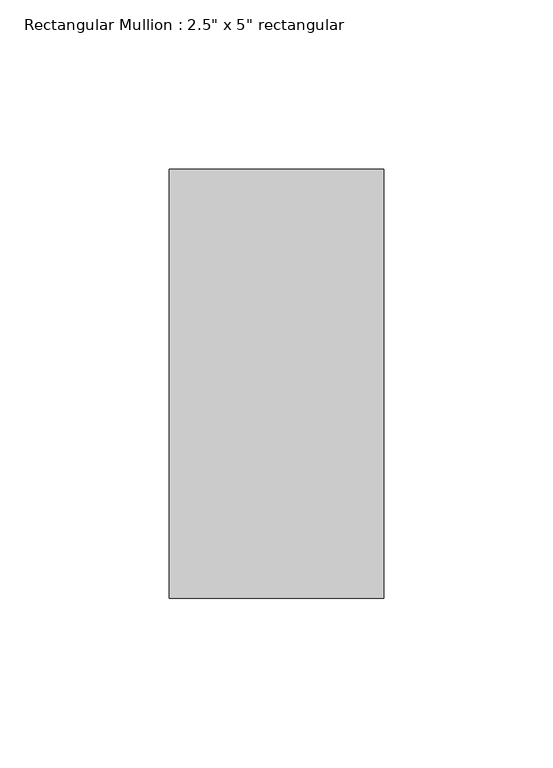
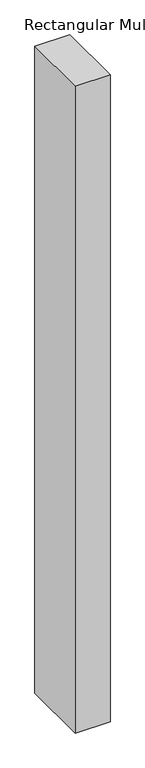
"""IFC4 building model written with IfcOpenShell, lengths in millimetres: member geometry."""

from ifc_helpers import new_model, si_unit, frame, origin, place, context, project, spatial, polyline, outline, extrude, source, transform, mapped, element, save


def member_71eb4692(model_context):
    return source(origin(), model_context, "Body", "SweptSolid", [
        extrude(outline(polyline([(0.0, 63.5), (0.0, -63.5), (-63.5, -63.5), (-63.5, 63.5), (0.0, 63.5)])), frame((0.0, 0.0, -1244.6), z_axis=(0.0, 0.0, 1.0), x_axis=(1.0, 0.0, 0.0)), (0.0, 0.0, 1.0), 1244.6),
    ])


if __name__ == "__main__":
    model = new_model("IFC4")
    model_context = context("Model", 3, world=origin())
    ifc_project = project(units=[si_unit("LENGTHUNIT", "METRE", prefix="MILLI")], contexts=[model_context])
    site = spatial("IfcSite", under=ifc_project)
    building = spatial("IfcBuilding", under=site)
    placement = place(None, origin())
    member_shape = member_71eb4692(model_context)
    element("IfcMember", 1, ObjectType="Rectangular Mullion : 2.5\" x 5\" rectangular", at=placement, inside=building, context=model_context, shape_type="MappedRepresentation", body=[
        mapped(member_shape, transform((0.0, 0.0, 0.0), x_axis=(1.0, 0.0, 0.0), y_axis=(0.0, 1.0, 0.0), z_axis=(0.0, 0.0, 1.0))),
    ])
    save(model, "model.ifc")

# Revit data of these elements
# Type "Rectangular Mullion : 2.5\" x 5\" rectangular"
#   built-in parameter 1007304 = 0.416667 (stored number, unit not read)
#   built-in parameter 1007301 = 0.104167 (stored number, unit not read)
#   built-in parameter 1007300 = 0.104167 (stored number, unit not read)
# Element 1 (IfcMember, "Rectangular Mullion : 2.5\" x 5\" rectangular")
#   Materials on its faces: "Iron, Ductile"
# Materials
#   "Iron, Ductile": class "Metal", colour RGB 0 0 0, transparency 0, Description = "Ductile cast iron", Cost = 0
